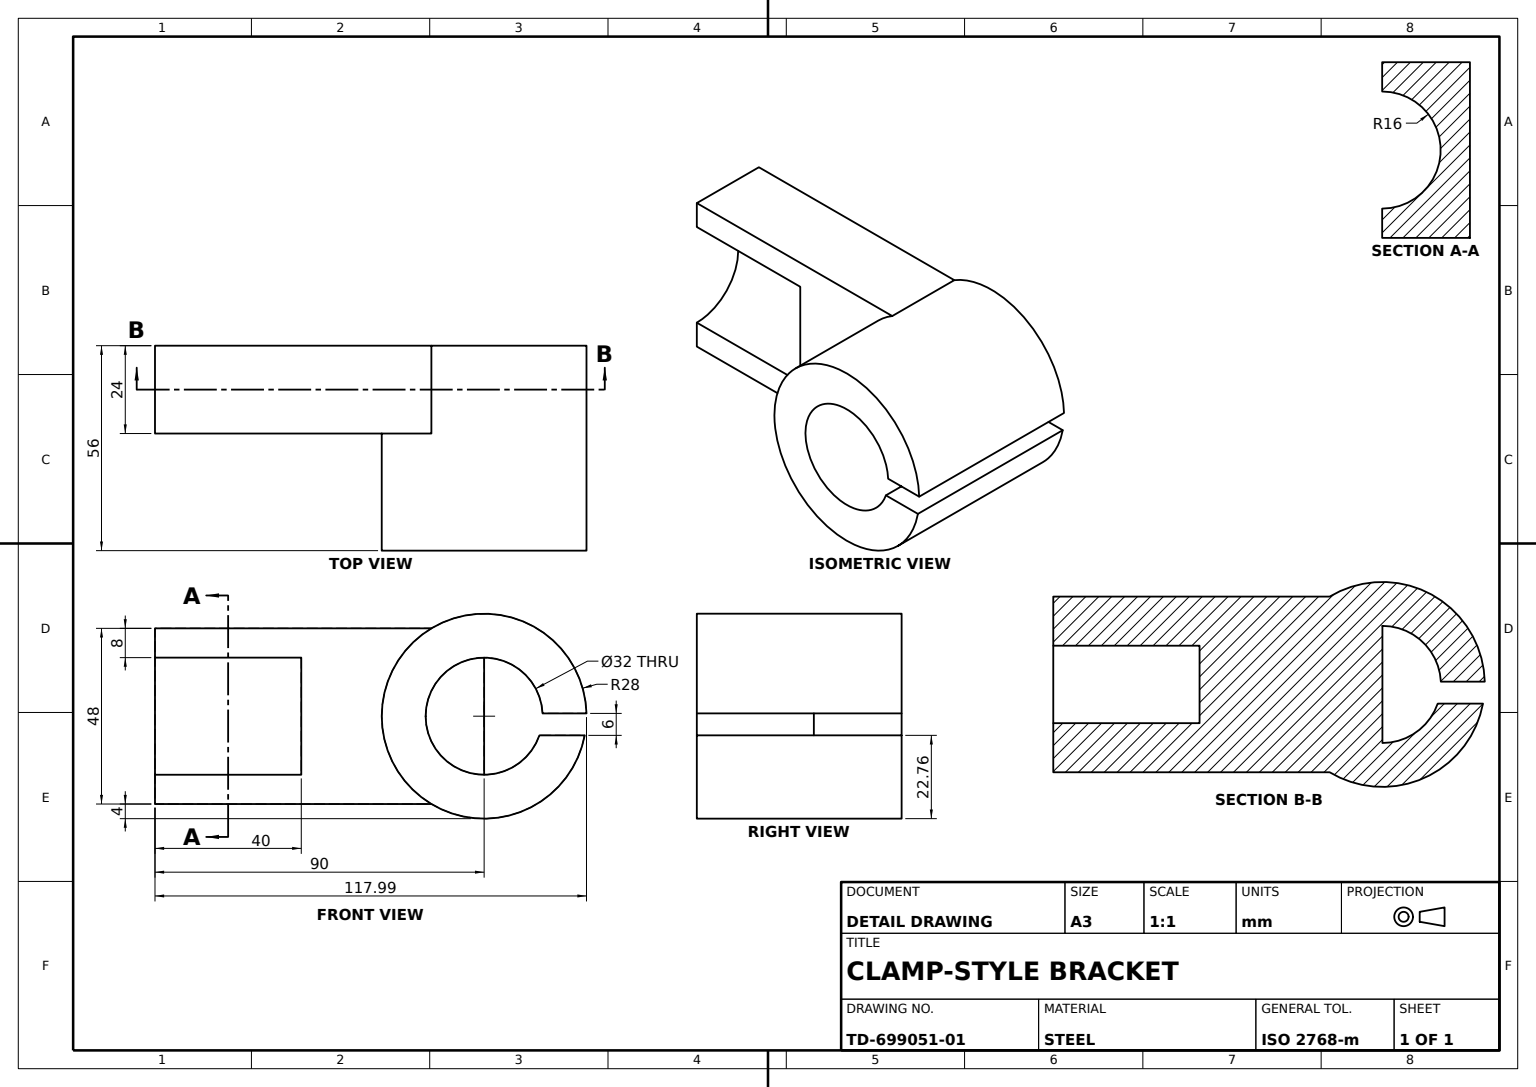
SolidWorks part; units mm, degrees
material "Plain Carbon Steel"
ref_plane "Front Plane" through (0, 0, 0) normal (0, 0, 1) x (1, 0, 0)
ref_plane "Top Plane" through (0, 0, 0) normal (0, 1, 0) x (1, 0, 0)
ref_plane "Right Plane" through (0, 0, 0) normal (1, 0, 0) x (0, 0, -1)
sketch "Base Block Sketch" plane through (0, 0, 0) normal (0, 0, 1) x (1, 0, 0)
  line L1 (-45, 24) -> (45, 24)
  line L2 (-45, 24) -> (-45, -24)
  line L3 (-45, -24) -> (45, -24)
  line L4 (45, 24) -> (45, -24)
  line L5 (-45, 24) -> (45, -24) construction
  line L6 (-45, -24) -> (45, 24) construction
  point P0 (0, 0)
  dimension "D1" = 48
  dimension "D2" = 90
extrude "Base Block" add sketch "Base Block Sketch" along normal mid plane 24
sketch "Cradle Cut Sketch" plane through (-45, 0, 0) normal (-1, 0, 0) x (0, 0, 1)
  line L0 (12, 24) -> (12, -24) construction
  line L1 (12, 16) -> (12, -16)
  line L2 (12, 24) -> (12, 16) construction
  line L3 (12, -16) -> (12, -24)
  arc A0 (12, 16) -> (12, -16) centre (12, 0) ccw
  point P3 (-4, 0)
  line M9 (12, -24) -> (12, 24)
  dimension "D3" = 16
  dimension "D1" = 32
  dimension "D2" = 8
extrude "Cradle Cut" cut sketch "Cradle Cut Sketch" against normal blind 40 contours A0 M9
sketch "Clamp Boss Sketch" plane through (0, 0, -12) normal (0, 0, -1) x (-1, 0, 0)
  line L0 (-45, -24) -> (-45, 24) construction
  circle A0 centre (-45, 0) radius 28
  circle A1 centre (-45, 0) radius 16
  dimension "D1" = 56
  dimension "D2" = 32
extrude "Clamp Boss Ø56" add sketch "Clamp Boss Sketch" against normal blind 56
sketch "Bore and Split Slot Sketch" plane through (0, 0, 44) normal (0, 0, 1) x (1, 0, 0)
  line L5 (57.6775, -2.2413) -> (57.6775, 0.7587)
  line L6 (57.6775, 0.7587) -> (76.6268, 0.7587)
  line L7 (76.6268, 0.7587) -> (76.6268, -5.2413)
  line L8 (76.6268, -5.2413) -> (57.6775, -5.2413)
  line L9 (57.6775, -5.2413) -> (57.6775, -2.2413)
  dimension "D1" = 3
  dimension "D2" = 3
  dimension "D3" = 18.9493
  dimension "D4" = 57.6775
  dimension "D5" = 5.2413
extrude "Bore and Split Slot Cut" cut sketch "Bore and Split Slot Sketch" against normal blind 56
